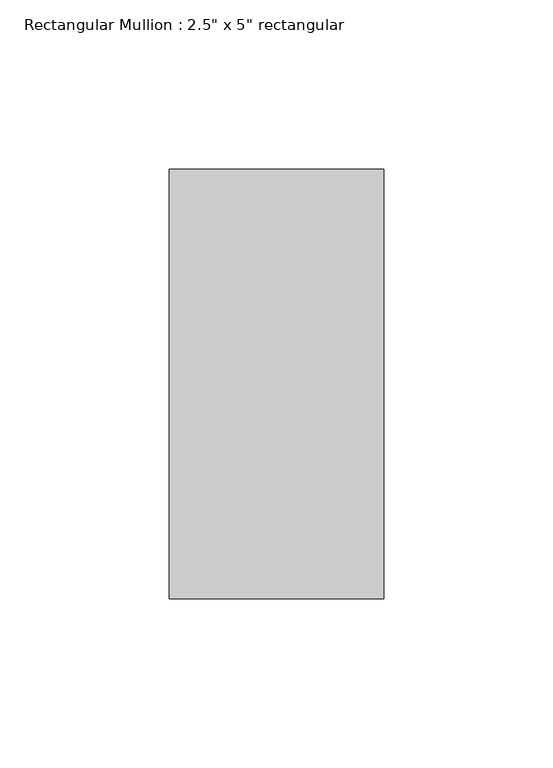
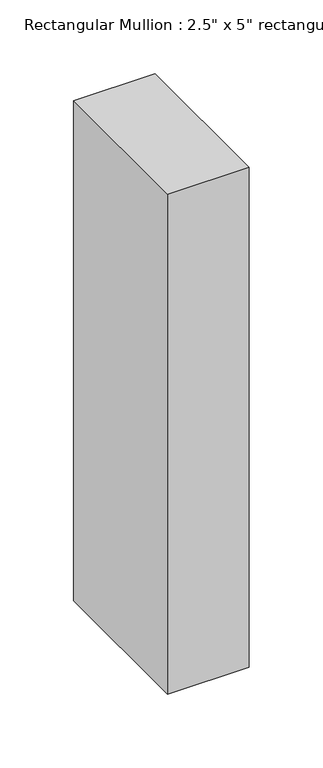
"""IFC4 building model written with IfcOpenShell, lengths in millimetres: member geometry."""

from ifc_helpers import new_model, si_unit, frame, origin, place, context, project, spatial, polyline, outline, extrude, source, transform, mapped, element, save


def member_dc106669(model_context):
    return source(origin(), model_context, "Body", "SweptSolid", [
        extrude(outline(polyline([(0.0, 63.5), (0.0, -63.5), (-63.5, -63.5), (-63.5, 63.5), (0.0, 63.5)])), frame((0.0, 0.0, -412.75), z_axis=(0.0, 0.0, 1.0), x_axis=(1.0, 0.0, 0.0)), (0.0, 0.0, 1.0), 412.75),
    ])


if __name__ == "__main__":
    model = new_model("IFC4")
    model_context = context("Model", 3, world=origin())
    ifc_project = project(units=[si_unit("LENGTHUNIT", "METRE", prefix="MILLI")], contexts=[model_context])
    site = spatial("IfcSite", under=ifc_project)
    building = spatial("IfcBuilding", under=site)
    placement = place(None, origin())
    member_shape = member_dc106669(model_context)
    element("IfcMember", 1, ObjectType="Rectangular Mullion : 2.5\" x 5\" rectangular", at=placement, inside=building, context=model_context, shape_type="MappedRepresentation", body=[
        mapped(member_shape, transform((0.0, 0.0, 0.0), x_axis=(1.0, 0.0, 0.0), y_axis=(0.0, 1.0, 0.0), z_axis=(0.0, 0.0, 1.0))),
    ])
    save(model, "model.ifc")

# Revit data of these elements
# Type "Rectangular Mullion : 2.5\" x 5\" rectangular"
#   built-in parameter 1007304 = 0.416667 (stored number, unit not read)
#   built-in parameter 1007301 = 0.104167 (stored number, unit not read)
#   built-in parameter 1007300 = 0.104167 (stored number, unit not read)
